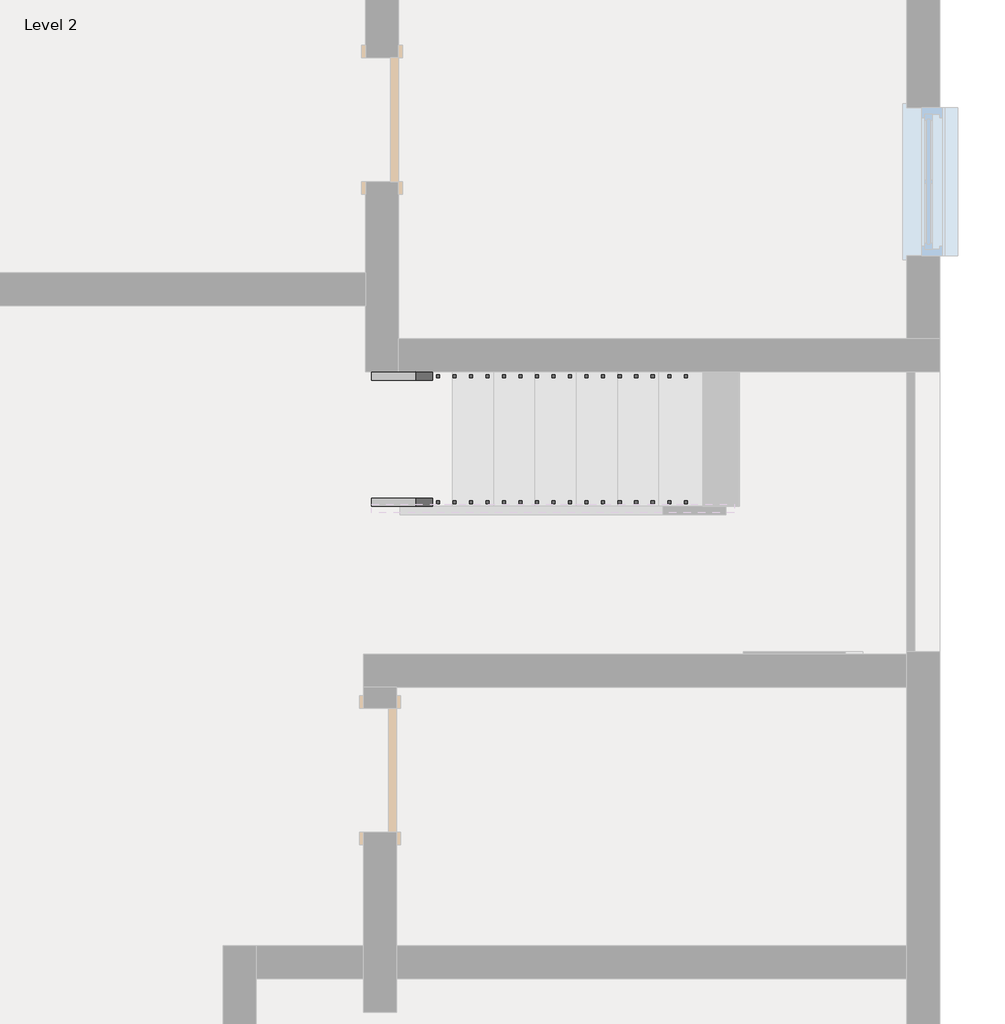
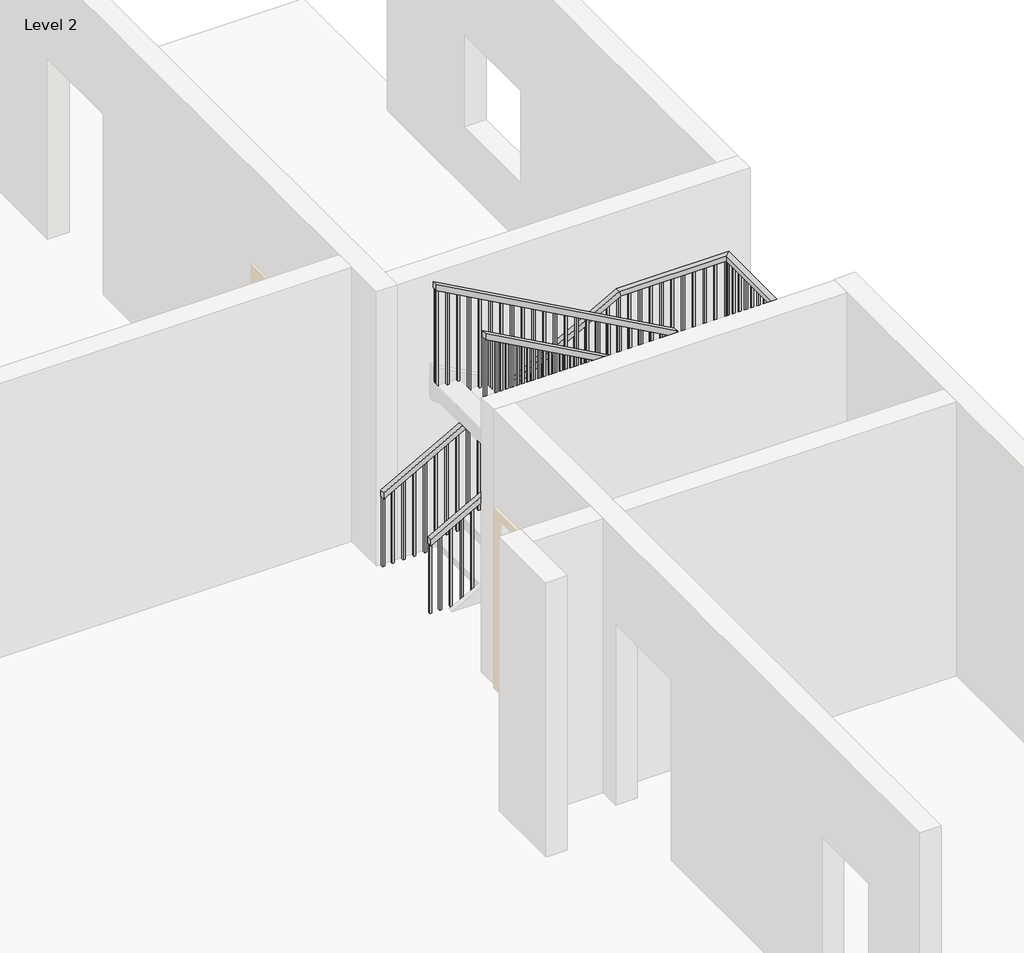
# One storey, part 3 of 4: 2 railings.
"""IFC4 building model written with IfcOpenShell, lengths in millimetres."""

from ifc_helpers import new_model, si_unit, frame, origin, place, context, project, spatial, polyline, outline, extrude, faceted_brep, element, save

model = new_model("IFC4")

# Units and contexts
model_context = context("Model", 3, world=origin())
ifc_project = project(units=[si_unit("LENGTHUNIT", "METRE", prefix="MILLI")], contexts=[model_context])

# Site, building, storey
site = spatial("IfcSite", under=ifc_project)
building = spatial("IfcBuilding", under=site)
storey = spatial("IfcBuildingStorey", under=building, Name="Level 2", Elevation=3048.0)

# Railings
placement = place(None, origin())
element("IfcRailing", 1, ObjectType="Handrail - Rectangular", at=placement, inside=storey, context=model_context, shape_type="SolidModel", body=[
    faceted_brep([(1537.1941283, 231.7547293, 4099.56), (1537.1941283, 231.7547293, 4041.4879132), (1537.1941283, 180.9547293, 4041.4879132), (1537.1941283, 180.9547293, 4099.56), (3765.8648053, 231.7547293, 5334.0), (3765.8648053, 180.9547293, 5334.0), (3765.8648053, 180.9547293, 5275.9279132), (3765.8648053, 231.7547293, 5275.9279132)], [[[0, 1, 2, 3]], [[4, 5, 6, 7]], [[1, 0, 4, 7]], [[2, 1, 7, 6]], [[3, 2, 6, 5]], [[0, 3, 5, 4]]]),
    faceted_brep([(3816.6648053, 231.7547293, 5334.0), (3816.6648053, 231.7547293, 5283.2), (3765.8648053, 231.7547293, 5283.2), (3765.8648053, 231.7547293, 5334.0), (3816.6648053, 142.8547293, 5334.0), (3765.8648053, 142.8547293, 5334.0), (3765.8648053, 92.0547293, 5283.2), (3816.6648053, 92.0547293, 5283.2)], [[[0, 1, 2, 3]], [[4, 5, 6, 7]], [[1, 0, 4, 7]], [[2, 1, 7, 6]], [[3, 2, 6, 5]], [[0, 3, 5, 4]]]),
    faceted_brep([(3816.6648053, 142.8547293, 5334.0), (3816.6648053, 92.0547293, 5283.2), (3765.8648053, 92.0547293, 5283.2), (3765.8648053, 142.8547293, 5334.0), (3816.6648053, 142.8547293, 5443.0223516), (3765.8648053, 142.8547293, 5413.0879132), (3765.8648053, 92.0547293, 5413.0879132), (3816.6648053, 92.0547293, 5443.0223516)], [[[0, 1, 2, 3]], [[4, 5, 6, 7]], [[1, 0, 4, 7]], [[2, 1, 7, 6]], [[3, 2, 6, 5]], [[0, 3, 5, 4]]]),
    faceted_brep([(3816.6648053, 92.0547293, 5443.0223516), (3765.8648053, 92.0547293, 5413.0879132), (3765.8648053, 142.8547293, 5413.0879132), (3816.6648053, 142.8547293, 5443.0223516), (1537.1941283, 92.0547293, 6705.6), (1537.1941283, 142.8547293, 6705.6), (1537.1941283, 142.8547293, 6647.5279132), (1537.1941283, 92.0547293, 6647.5279132)], [[[0, 1, 2, 3]], [[4, 5, 6, 7]], [[1, 0, 4, 7]], [[2, 1, 7, 6]], [[3, 2, 6, 5]], [[0, 3, 5, 4]]]),
    extrude(outline(polyline([(6631.7556667, 1565.5898053), (6642.3072849, 1546.5398053), (5654.04, 1546.5398053), (5654.04, 1565.5898053), (6631.7556667, 1565.5898053)])), frame((0.0, 107.9297293, 0.0), z_axis=(0.0, 1.0, 0.0), x_axis=(0.0, 0.0, 1.0)), (0.0, 0.0, 1.0), 19.05),
    extrude(outline(polyline([(6575.4803699, 1667.1898053), (6586.031988, 1648.1398053), (5654.04, 1648.1398053), (5654.04, 1667.1898053), (6575.4803699, 1667.1898053)])), frame((0.0, 107.9297293, 0.0), z_axis=(0.0, 1.0, 0.0), x_axis=(0.0, 0.0, 1.0)), (0.0, 0.0, 1.0), 19.05),
    extrude(outline(polyline([(6519.1609284, 1768.7898053), (6529.7125465, 1749.7398053), (5654.04, 1749.7398053), (5654.04, 1768.7898053), (6519.1609284, 1768.7898053)])), frame((0.0, 107.9297293, 0.0), z_axis=(0.0, 1.0, 0.0), x_axis=(0.0, 0.0, 1.0)), (0.0, 0.0, 1.0), 19.05),
    extrude(outline(polyline([(6462.9297761, 1870.3898053), (6473.4813943, 1851.3398053), (5516.88, 1851.3398053), (5516.88, 1870.3898053), (6462.9297761, 1870.3898053)])), frame((0.0, 107.9297293, 0.0), z_axis=(0.0, 1.0, 0.0), x_axis=(0.0, 0.0, 1.0)), (0.0, 0.0, 1.0), 19.05),
    extrude(outline(polyline([(6406.6544792, 1971.9898053), (6417.2060974, 1952.9398053), (5516.88, 1952.9398053), (5516.88, 1971.9898053), (6406.6544792, 1971.9898053)])), frame((0.0, 107.9297293, 0.0), z_axis=(0.0, 1.0, 0.0), x_axis=(0.0, 0.0, 1.0)), (0.0, 0.0, 1.0), 19.05),
    extrude(outline(polyline([(6350.3791823, 2073.5898053), (6360.9308005, 2054.5398053), (5379.72, 2054.5398053), (5379.72, 2073.5898053), (6350.3791823, 2073.5898053)])), frame((0.0, 107.9297293, 0.0), z_axis=(0.0, 1.0, 0.0), x_axis=(0.0, 0.0, 1.0)), (0.0, 0.0, 1.0), 19.05),
    extrude(outline(polyline([(6294.1038855, 2175.1898053), (6304.6555036, 2156.1398053), (5379.72, 2156.1398053), (5379.72, 2175.1898053), (6294.1038855, 2175.1898053)])), frame((0.0, 107.9297293, 0.0), z_axis=(0.0, 1.0, 0.0), x_axis=(0.0, 0.0, 1.0)), (0.0, 0.0, 1.0), 19.05),
    extrude(outline(polyline([(6237.8285886, 2276.7898053), (6248.3802067, 2257.7398053), (5379.72, 2257.7398053), (5379.72, 2276.7898053), (6237.8285886, 2276.7898053)])), frame((0.0, 107.9297293, 0.0), z_axis=(0.0, 1.0, 0.0), x_axis=(0.0, 0.0, 1.0)), (0.0, 0.0, 1.0), 19.05),
    extrude(outline(polyline([(6181.5532917, 2378.3898053), (6192.1049099, 2359.3398053), (5242.56, 2359.3398053), (5242.56, 2378.3898053), (6181.5532917, 2378.3898053)])), frame((0.0, 107.9297293, 0.0), z_axis=(0.0, 1.0, 0.0), x_axis=(0.0, 0.0, 1.0)), (0.0, 0.0, 1.0), 19.05),
    extrude(outline(polyline([(6125.2779948, 2479.9898053), (6135.829613, 2460.9398053), (5242.56, 2460.9398053), (5242.56, 2479.9898053), (6125.2779948, 2479.9898053)])), frame((0.0, 107.9297293, 0.0), z_axis=(0.0, 1.0, 0.0), x_axis=(0.0, 0.0, 1.0)), (0.0, 0.0, 1.0), 19.05),
    extrude(outline(polyline([(6069.0026979, 2581.5898053), (6079.5543161, 2562.5398053), (5105.4, 2562.5398053), (5105.4, 2581.5898053), (6069.0026979, 2581.5898053)])), frame((0.0, 107.9297293, 0.0), z_axis=(0.0, 1.0, 0.0), x_axis=(0.0, 0.0, 1.0)), (0.0, 0.0, 1.0), 19.05),
    extrude(outline(polyline([(6012.727401, 2683.1898053), (6023.2790192, 2664.1398053), (5105.4, 2664.1398053), (5105.4, 2683.1898053), (6012.727401, 2683.1898053)])), frame((0.0, 107.9297293, 0.0), z_axis=(0.0, 1.0, 0.0), x_axis=(0.0, 0.0, 1.0)), (0.0, 0.0, 1.0), 19.05),
    extrude(outline(polyline([(5956.4962488, 2784.7898053), (5967.0478669, 2765.7398053), (5105.4, 2765.7398053), (5105.4, 2784.7898053), (5956.4962488, 2784.7898053)])), frame((0.0, 107.9297293, 0.0), z_axis=(0.0, 1.0, 0.0), x_axis=(0.0, 0.0, 1.0)), (0.0, 0.0, 1.0), 19.05),
    extrude(outline(polyline([(5900.2209519, 2886.3898053), (5910.77257, 2867.3398053), (4968.24, 2867.3398053), (4968.24, 2886.3898053), (5900.2209519, 2886.3898053)])), frame((0.0, 107.9297293, 0.0), z_axis=(0.0, 1.0, 0.0), x_axis=(0.0, 0.0, 1.0)), (0.0, 0.0, 1.0), 19.05),
    extrude(outline(polyline([(5843.945655, 2987.9898053), (5854.4972732, 2968.9398053), (4968.24, 2968.9398053), (4968.24, 2987.9898053), (5843.945655, 2987.9898053)])), frame((0.0, 107.9297293, 0.0), z_axis=(0.0, 1.0, 0.0), x_axis=(0.0, 0.0, 1.0)), (0.0, 0.0, 1.0), 19.05),
    extrude(outline(polyline([(5787.6703581, 3089.5898053), (5798.2219763, 3070.5398053), (4831.08, 3070.5398053), (4831.08, 3089.5898053), (5787.6703581, 3089.5898053)])), frame((0.0, 107.9297293, 0.0), z_axis=(0.0, 1.0, 0.0), x_axis=(0.0, 0.0, 1.0)), (0.0, 0.0, 1.0), 19.05),
    extrude(outline(polyline([(5731.3950612, 3191.1898053), (5741.9466794, 3172.1398053), (4831.08, 3172.1398053), (4831.08, 3191.1898053), (5731.3950612, 3191.1898053)])), frame((0.0, 107.9297293, 0.0), z_axis=(0.0, 1.0, 0.0), x_axis=(0.0, 0.0, 1.0)), (0.0, 0.0, 1.0), 19.05),
    extrude(outline(polyline([(5675.1197643, 3292.7898053), (5685.6713825, 3273.7398053), (4831.08, 3273.7398053), (4831.08, 3292.7898053), (5675.1197643, 3292.7898053)])), frame((0.0, 107.9297293, 0.0), z_axis=(0.0, 1.0, 0.0), x_axis=(0.0, 0.0, 1.0)), (0.0, 0.0, 1.0), 19.05),
    extrude(outline(polyline([(5618.8444675, 3394.3898053), (5629.3960856, 3375.3398053), (4693.92, 3375.3398053), (4693.92, 3394.3898053), (5618.8444675, 3394.3898053)])), frame((0.0, 107.9297293, 0.0), z_axis=(0.0, 1.0, 0.0), x_axis=(0.0, 0.0, 1.0)), (0.0, 0.0, 1.0), 19.05),
    extrude(outline(polyline([(5562.5691706, 3495.9898053), (5573.1207888, 3476.9398053), (4693.92, 3476.9398053), (4693.92, 3495.9898053), (5562.5691706, 3495.9898053)])), frame((0.0, 107.9297293, 0.0), z_axis=(0.0, 1.0, 0.0), x_axis=(0.0, 0.0, 1.0)), (0.0, 0.0, 1.0), 19.05),
    extrude(outline(polyline([(5506.2938737, 3597.5898053), (5516.8454919, 3578.5398053), (4556.76, 3578.5398053), (4556.76, 3597.5898053), (5506.2938737, 3597.5898053)])), frame((0.0, 107.9297293, 0.0), z_axis=(0.0, 1.0, 0.0), x_axis=(0.0, 0.0, 1.0)), (0.0, 0.0, 1.0), 19.05),
    extrude(outline(polyline([(5450.0185768, 3699.1898053), (5460.570195, 3680.1398053), (4556.76, 3680.1398053), (4556.76, 3699.1898053), (5450.0185768, 3699.1898053)])), frame((0.0, 107.9297293, 0.0), z_axis=(0.0, 1.0, 0.0), x_axis=(0.0, 0.0, 1.0)), (0.0, 0.0, 1.0), 19.05),
    extrude(outline(polyline([(5284.8202537, 3781.9191283), (5274.2686355, 3762.8691283), (4419.6, 3762.8691283), (4419.6, 3781.9191283), (5284.8202537, 3781.9191283)])), frame((0.0, 196.8297293, 0.0), z_axis=(0.0, 1.0, 0.0), x_axis=(0.0, 0.0, 1.0)), (0.0, 0.0, 1.0), 19.05),
    extrude(outline(polyline([(5228.5449568, 3680.3191283), (5217.9933387, 3661.2691283), (4282.44, 3661.2691283), (4282.44, 3680.3191283), (5228.5449568, 3680.3191283)])), frame((0.0, 196.8297293, 0.0), z_axis=(0.0, 1.0, 0.0), x_axis=(0.0, 0.0, 1.0)), (0.0, 0.0, 1.0), 19.05),
    extrude(outline(polyline([(5172.2696599, 3578.7191283), (5161.7180418, 3559.6691283), (4282.44, 3559.6691283), (4282.44, 3578.7191283), (5172.2696599, 3578.7191283)])), frame((0.0, 196.8297293, 0.0), z_axis=(0.0, 1.0, 0.0), x_axis=(0.0, 0.0, 1.0)), (0.0, 0.0, 1.0), 19.05),
    extrude(outline(polyline([(5115.9943631, 3477.1191283), (5105.4427449, 3458.0691283), (4145.28, 3458.0691283), (4145.28, 3477.1191283), (5115.9943631, 3477.1191283)])), frame((0.0, 196.8297293, 0.0), z_axis=(0.0, 1.0, 0.0), x_axis=(0.0, 0.0, 1.0)), (0.0, 0.0, 1.0), 19.05),
    extrude(outline(polyline([(5059.7190662, 3375.5191283), (5049.167448, 3356.4691283), (4145.28, 3356.4691283), (4145.28, 3375.5191283), (5059.7190662, 3375.5191283)])), frame((0.0, 196.8297293, 0.0), z_axis=(0.0, 1.0, 0.0), x_axis=(0.0, 0.0, 1.0)), (0.0, 0.0, 1.0), 19.05),
    extrude(outline(polyline([(5003.4437693, 3273.9191283), (4992.8921511, 3254.8691283), (4008.12, 3254.8691283), (4008.12, 3273.9191283), (5003.4437693, 3273.9191283)])), frame((0.0, 196.8297293, 0.0), z_axis=(0.0, 1.0, 0.0), x_axis=(0.0, 0.0, 1.0)), (0.0, 0.0, 1.0), 19.05),
    extrude(outline(polyline([(4947.1684724, 3172.3191283), (4936.6168543, 3153.2691283), (4008.12, 3153.2691283), (4008.12, 3172.3191283), (4947.1684724, 3172.3191283)])), frame((0.0, 196.8297293, 0.0), z_axis=(0.0, 1.0, 0.0), x_axis=(0.0, 0.0, 1.0)), (0.0, 0.0, 1.0), 19.05),
    extrude(outline(polyline([(4890.8931755, 3070.7191283), (4880.3415574, 3051.6691283), (4008.12, 3051.6691283), (4008.12, 3070.7191283), (4890.8931755, 3070.7191283)])), frame((0.0, 196.8297293, 0.0), z_axis=(0.0, 1.0, 0.0), x_axis=(0.0, 0.0, 1.0)), (0.0, 0.0, 1.0), 19.05),
    extrude(outline(polyline([(4834.6178787, 2969.1191283), (4824.0662605, 2950.0691283), (3870.96, 2950.0691283), (3870.96, 2969.1191283), (4834.6178787, 2969.1191283)])), frame((0.0, 196.8297293, 0.0), z_axis=(0.0, 1.0, 0.0), x_axis=(0.0, 0.0, 1.0)), (0.0, 0.0, 1.0), 19.05),
    extrude(outline(polyline([(4778.3425818, 2867.5191283), (4767.7909636, 2848.4691283), (3870.96, 2848.4691283), (3870.96, 2867.5191283), (4778.3425818, 2867.5191283)])), frame((0.0, 196.8297293, 0.0), z_axis=(0.0, 1.0, 0.0), x_axis=(0.0, 0.0, 1.0)), (0.0, 0.0, 1.0), 19.05),
    extrude(outline(polyline([(4722.0672849, 2765.9191283), (4711.5156667, 2746.8691283), (3733.8, 2746.8691283), (3733.8, 2765.9191283), (4722.0672849, 2765.9191283)])), frame((0.0, 196.8297293, 0.0), z_axis=(0.0, 1.0, 0.0), x_axis=(0.0, 0.0, 1.0)), (0.0, 0.0, 1.0), 19.05),
    extrude(outline(polyline([(4665.791988, 2664.3191283), (4655.2403699, 2645.2691283), (3733.8, 2645.2691283), (3733.8, 2664.3191283), (4665.791988, 2664.3191283)])), frame((0.0, 196.8297293, 0.0), z_axis=(0.0, 1.0, 0.0), x_axis=(0.0, 0.0, 1.0)), (0.0, 0.0, 1.0), 19.05),
    extrude(outline(polyline([(4609.4725465, 2562.7191283), (4598.9209284, 2543.6691283), (3733.8, 2543.6691283), (3733.8, 2562.7191283), (4609.4725465, 2562.7191283)])), frame((0.0, 196.8297293, 0.0), z_axis=(0.0, 1.0, 0.0), x_axis=(0.0, 0.0, 1.0)), (0.0, 0.0, 1.0), 19.05),
    extrude(outline(polyline([(4553.2413943, 2461.1191283), (4542.6897761, 2442.0691283), (3596.64, 2442.0691283), (3596.64, 2461.1191283), (4553.2413943, 2461.1191283)])), frame((0.0, 196.8297293, 0.0), z_axis=(0.0, 1.0, 0.0), x_axis=(0.0, 0.0, 1.0)), (0.0, 0.0, 1.0), 19.05),
    extrude(outline(polyline([(4496.9660974, 2359.5191283), (4486.4144792, 2340.4691283), (3596.64, 2340.4691283), (3596.64, 2359.5191283), (4496.9660974, 2359.5191283)])), frame((0.0, 196.8297293, 0.0), z_axis=(0.0, 1.0, 0.0), x_axis=(0.0, 0.0, 1.0)), (0.0, 0.0, 1.0), 19.05),
    extrude(outline(polyline([(4440.6908005, 2257.9191283), (4430.1391823, 2238.8691283), (3459.48, 2238.8691283), (3459.48, 2257.9191283), (4440.6908005, 2257.9191283)])), frame((0.0, 196.8297293, 0.0), z_axis=(0.0, 1.0, 0.0), x_axis=(0.0, 0.0, 1.0)), (0.0, 0.0, 1.0), 19.05),
    extrude(outline(polyline([(4384.4155036, 2156.3191283), (4373.8638855, 2137.2691283), (3459.48, 2137.2691283), (3459.48, 2156.3191283), (4384.4155036, 2156.3191283)])), frame((0.0, 196.8297293, 0.0), z_axis=(0.0, 1.0, 0.0), x_axis=(0.0, 0.0, 1.0)), (0.0, 0.0, 1.0), 19.05),
    extrude(outline(polyline([(4328.1402067, 2054.7191283), (4317.5885886, 2035.6691283), (3459.48, 2035.6691283), (3459.48, 2054.7191283), (4328.1402067, 2054.7191283)])), frame((0.0, 196.8297293, 0.0), z_axis=(0.0, 1.0, 0.0), x_axis=(0.0, 0.0, 1.0)), (0.0, 0.0, 1.0), 19.05),
    extrude(outline(polyline([(4271.8649099, 1953.1191283), (4261.3132917, 1934.0691283), (3322.32, 1934.0691283), (3322.32, 1953.1191283), (4271.8649099, 1953.1191283)])), frame((0.0, 196.8297293, 0.0), z_axis=(0.0, 1.0, 0.0), x_axis=(0.0, 0.0, 1.0)), (0.0, 0.0, 1.0), 19.05),
    extrude(outline(polyline([(4215.589613, 1851.5191283), (4205.0379948, 1832.4691283), (3322.32, 1832.4691283), (3322.32, 1851.5191283), (4215.589613, 1851.5191283)])), frame((0.0, 196.8297293, 0.0), z_axis=(0.0, 1.0, 0.0), x_axis=(0.0, 0.0, 1.0)), (0.0, 0.0, 1.0), 19.05),
    extrude(outline(polyline([(4159.3143161, 1749.9191283), (4148.7626979, 1730.8691283), (3185.16, 1730.8691283), (3185.16, 1749.9191283), (4159.3143161, 1749.9191283)])), frame((0.0, 196.8297293, 0.0), z_axis=(0.0, 1.0, 0.0), x_axis=(0.0, 0.0, 1.0)), (0.0, 0.0, 1.0), 19.05),
    extrude(outline(polyline([(4103.0390192, 1648.3191283), (4092.487401, 1629.2691283), (3185.16, 1629.2691283), (3185.16, 1648.3191283), (4103.0390192, 1648.3191283)])), frame((0.0, 196.8297293, 0.0), z_axis=(0.0, 1.0, 0.0), x_axis=(0.0, 0.0, 1.0)), (0.0, 0.0, 1.0), 19.05),
    extrude(outline(polyline([(3781.7398053, 126.9797293), (3800.7898053, 126.9797293), (3800.7898053, 107.9297293), (3781.7398053, 107.9297293), (3781.7398053, 126.9797293)])), frame((0.0, 0.0, 4419.6), z_axis=(0.0, 0.0, 1.0), x_axis=(1.0, 0.0, 0.0)), (0.0, 0.0, 1.0), 863.6),
    extrude(outline(polyline([(5295.2725465, 3800.7898053), (5284.7209284, 3781.7398053), (4419.6, 3781.7398053), (4419.6, 3800.7898053), (5295.2725465, 3800.7898053)])), frame((0.0, 196.8297293, 0.0), z_axis=(0.0, 1.0, 0.0), x_axis=(0.0, 0.0, 1.0)), (0.0, 0.0, 1.0), 19.05),
    extrude(outline(polyline([(6636.9762951, 1556.2441283), (6647.5279132, 1537.1941283), (5654.04, 1537.1941283), (5654.04, 1556.2441283), (6636.9762951, 1556.2441283)])), frame((0.0, 107.9297293, 0.0), z_axis=(0.0, 1.0, 0.0), x_axis=(0.0, 0.0, 1.0)), (0.0, 0.0, 1.0), 19.05),
    extrude(outline(polyline([(4052.0395314, 1556.2441283), (4041.4879132, 1537.1941283), (3185.16, 1537.1941283), (3185.16, 1556.2441283), (4052.0395314, 1556.2441283)])), frame((0.0, 196.8297293, 0.0), z_axis=(0.0, 1.0, 0.0), x_axis=(0.0, 0.0, 1.0)), (0.0, 0.0, 1.0), 19.05),
])
element("IfcRailing", 2, ObjectType="Handrail - Rectangular", at=placement, inside=storey, context=model_context, shape_type="SolidModel", body=[
    faceted_brep([(1537.1941283, 1006.4547293, 4099.56), (1537.1941283, 1006.4547293, 4041.4879132), (1537.1941283, 955.6547293, 4041.4879132), (1537.1941283, 955.6547293, 4099.56), (3765.8648053, 1006.4547293, 5334.0), (3778.9939056, 1006.4547293, 5283.2), (3778.9939056, 955.6547293, 5283.2), (3765.8648053, 955.6547293, 5334.0), (4826.4941283, 1006.4547293, 5334.0), (4826.4941283, 1006.4547293, 5283.2), (4775.6941283, 955.6547293, 5283.2), (4775.6941283, 955.6547293, 5334.0), (4826.4941283, -714.2964201, 5334.0), (4826.4941283, -714.2964201, 5283.2), (4775.6941283, -663.4964201, 5283.2), (4775.6941283, -663.4964201, 5334.0), (4013.4948805, -714.2964201, 5334.0), (4000.3657803, -714.2964201, 5283.2), (4000.3657803, -663.4964201, 5283.2), (4013.4948805, -663.4964201, 5334.0), (1537.1941283, -714.2964201, 6705.6), (1537.1941283, -663.4964201, 6705.6), (1537.1941283, -663.4964201, 6647.5279132), (1537.1941283, -714.2964201, 6647.5279132)], [[[0, 1, 2, 3]], [[1, 0, 4, 5]], [[2, 1, 5, 6]], [[3, 2, 6, 7]], [[0, 3, 7, 4]], [[5, 4, 8, 9]], [[6, 5, 9, 10]], [[7, 6, 10, 11]], [[4, 7, 11, 8]], [[9, 8, 12, 13]], [[10, 9, 13, 14]], [[11, 10, 14, 15]], [[8, 11, 15, 12]], [[13, 12, 16, 17]], [[14, 13, 17, 18]], [[15, 14, 18, 19]], [[12, 15, 19, 16]], [[20, 21, 22, 23]], [[17, 16, 20, 23]], [[18, 17, 23, 22]], [[19, 18, 22, 21]], [[16, 19, 21, 20]]]),
    extrude(outline(polyline([(6645.7693102, 1540.3691283), (5654.04, 1540.3691283), (5654.04, 1559.4191283), (6635.2176921, 1559.4191283), (6645.7693102, 1540.3691283)])), frame((0.0, -698.4214201, 0.0), z_axis=(0.0, 1.0, 0.0), x_axis=(0.0, 0.0, 1.0)), (0.0, 0.0, 1.0), 19.05),
    extrude(outline(polyline([(6589.4940133, 1641.9691283), (5654.04, 1641.9691283), (5654.04, 1661.0191283), (6578.9423952, 1661.0191283), (6589.4940133, 1641.9691283)])), frame((0.0, -698.4214201, 0.0), z_axis=(0.0, 1.0, 0.0), x_axis=(0.0, 0.0, 1.0)), (0.0, 0.0, 1.0), 19.05),
    extrude(outline(polyline([(6533.2187165, 1743.5691283), (5654.04, 1743.5691283), (5654.04, 1762.6191283), (6522.6670983, 1762.6191283), (6533.2187165, 1743.5691283)])), frame((0.0, -698.4214201, 0.0), z_axis=(0.0, 1.0, 0.0), x_axis=(0.0, 0.0, 1.0)), (0.0, 0.0, 1.0), 19.05),
    extrude(outline(polyline([(6476.9434196, 1845.1691283), (5516.88, 1845.1691283), (5516.88, 1864.2191283), (6466.3918014, 1864.2191283), (6476.9434196, 1845.1691283)])), frame((0.0, -698.4214201, 0.0), z_axis=(0.0, 1.0, 0.0), x_axis=(0.0, 0.0, 1.0)), (0.0, 0.0, 1.0), 19.05),
    extrude(outline(polyline([(6420.6681227, 1946.7691283), (5516.88, 1946.7691283), (5516.88, 1965.8191283), (6410.1165045, 1965.8191283), (6420.6681227, 1946.7691283)])), frame((0.0, -698.4214201, 0.0), z_axis=(0.0, 1.0, 0.0), x_axis=(0.0, 0.0, 1.0)), (0.0, 0.0, 1.0), 19.05),
    extrude(outline(polyline([(6364.3928258, 2048.3691283), (5379.72, 2048.3691283), (5379.72, 2067.4191283), (6353.8412076, 2067.4191283), (6364.3928258, 2048.3691283)])), frame((0.0, -698.4214201, 0.0), z_axis=(0.0, 1.0, 0.0), x_axis=(0.0, 0.0, 1.0)), (0.0, 0.0, 1.0), 19.05),
    extrude(outline(polyline([(6308.1175289, 2149.9691283), (5379.72, 2149.9691283), (5379.72, 2169.0191283), (6297.5659108, 2169.0191283), (6308.1175289, 2149.9691283)])), frame((0.0, -698.4214201, 0.0), z_axis=(0.0, 1.0, 0.0), x_axis=(0.0, 0.0, 1.0)), (0.0, 0.0, 1.0), 19.05),
    extrude(outline(polyline([(6251.8422321, 2251.5691283), (5379.72, 2251.5691283), (5379.72, 2270.6191283), (6241.2906139, 2270.6191283), (6251.8422321, 2251.5691283)])), frame((0.0, -698.4214201, 0.0), z_axis=(0.0, 1.0, 0.0), x_axis=(0.0, 0.0, 1.0)), (0.0, 0.0, 1.0), 19.05),
    extrude(outline(polyline([(6195.5669352, 2353.1691283), (5242.56, 2353.1691283), (5242.56, 2372.2191283), (6185.015317, 2372.2191283), (6195.5669352, 2353.1691283)])), frame((0.0, -698.4214201, 0.0), z_axis=(0.0, 1.0, 0.0), x_axis=(0.0, 0.0, 1.0)), (0.0, 0.0, 1.0), 19.05),
    extrude(outline(polyline([(6139.2916383, 2454.7691283), (5242.56, 2454.7691283), (5242.56, 2473.8191283), (6128.7400201, 2473.8191283), (6139.2916383, 2454.7691283)])), frame((0.0, -698.4214201, 0.0), z_axis=(0.0, 1.0, 0.0), x_axis=(0.0, 0.0, 1.0)), (0.0, 0.0, 1.0), 19.05),
    extrude(outline(polyline([(6083.0163414, 2556.3691283), (5105.4, 2556.3691283), (5105.4, 2575.4191283), (6072.4647232, 2575.4191283), (6083.0163414, 2556.3691283)])), frame((0.0, -698.4214201, 0.0), z_axis=(0.0, 1.0, 0.0), x_axis=(0.0, 0.0, 1.0)), (0.0, 0.0, 1.0), 19.05),
    extrude(outline(polyline([(6026.7410445, 2657.9691283), (5105.4, 2657.9691283), (5105.4, 2677.0191283), (6016.1894264, 2677.0191283), (6026.7410445, 2657.9691283)])), frame((0.0, -698.4214201, 0.0), z_axis=(0.0, 1.0, 0.0), x_axis=(0.0, 0.0, 1.0)), (0.0, 0.0, 1.0), 19.05),
    extrude(outline(polyline([(5970.4657476, 2759.5691283), (5105.4, 2759.5691283), (5105.4, 2778.6191283), (5959.9141295, 2778.6191283), (5970.4657476, 2759.5691283)])), frame((0.0, -698.4214201, 0.0), z_axis=(0.0, 1.0, 0.0), x_axis=(0.0, 0.0, 1.0)), (0.0, 0.0, 1.0), 19.05),
    extrude(outline(polyline([(5914.3449568, 2861.1691283), (4968.24, 2861.1691283), (4968.24, 2880.2191283), (5903.7933387, 2880.2191283), (5914.3449568, 2861.1691283)])), frame((0.0, -698.4214201, 0.0), z_axis=(0.0, 1.0, 0.0), x_axis=(0.0, 0.0, 1.0)), (0.0, 0.0, 1.0), 19.05),
    extrude(outline(polyline([(5858.0696599, 2962.7691283), (4968.24, 2962.7691283), (4968.24, 2981.8191283), (5847.5180418, 2981.8191283), (5858.0696599, 2962.7691283)])), frame((0.0, -698.4214201, 0.0), z_axis=(0.0, 1.0, 0.0), x_axis=(0.0, 0.0, 1.0)), (0.0, 0.0, 1.0), 19.05),
    extrude(outline(polyline([(5801.7943631, 3064.3691283), (4831.08, 3064.3691283), (4831.08, 3083.4191283), (5791.2427449, 3083.4191283), (5801.7943631, 3064.3691283)])), frame((0.0, -698.4214201, 0.0), z_axis=(0.0, 1.0, 0.0), x_axis=(0.0, 0.0, 1.0)), (0.0, 0.0, 1.0), 19.05),
    extrude(outline(polyline([(5745.5190662, 3165.9691283), (4831.08, 3165.9691283), (4831.08, 3185.0191283), (5734.967448, 3185.0191283), (5745.5190662, 3165.9691283)])), frame((0.0, -698.4214201, 0.0), z_axis=(0.0, 1.0, 0.0), x_axis=(0.0, 0.0, 1.0)), (0.0, 0.0, 1.0), 19.05),
    extrude(outline(polyline([(5689.0892632, 3267.5691283), (4831.08, 3267.5691283), (4831.08, 3286.6191283), (5678.5376451, 3286.6191283), (5689.0892632, 3267.5691283)])), frame((0.0, -698.4214201, 0.0), z_axis=(0.0, 1.0, 0.0), x_axis=(0.0, 0.0, 1.0)), (0.0, 0.0, 1.0), 19.05),
    extrude(outline(polyline([(5632.9684724, 3369.1691283), (4693.92, 3369.1691283), (4693.92, 3388.2191283), (5622.4168543, 3388.2191283), (5632.9684724, 3369.1691283)])), frame((0.0, -698.4214201, 0.0), z_axis=(0.0, 1.0, 0.0), x_axis=(0.0, 0.0, 1.0)), (0.0, 0.0, 1.0), 19.05),
    extrude(outline(polyline([(5576.6931755, 3470.7691283), (4693.92, 3470.7691283), (4693.92, 3489.8191283), (5566.1415574, 3489.8191283), (5576.6931755, 3470.7691283)])), frame((0.0, -698.4214201, 0.0), z_axis=(0.0, 1.0, 0.0), x_axis=(0.0, 0.0, 1.0)), (0.0, 0.0, 1.0), 19.05),
    extrude(outline(polyline([(5520.4178787, 3572.3691283), (4556.76, 3572.3691283), (4556.76, 3591.4191283), (5509.8662605, 3591.4191283), (5520.4178787, 3572.3691283)])), frame((0.0, -698.4214201, 0.0), z_axis=(0.0, 1.0, 0.0), x_axis=(0.0, 0.0, 1.0)), (0.0, 0.0, 1.0), 19.05),
    extrude(outline(polyline([(5464.1425818, 3673.9691283), (4556.76, 3673.9691283), (4556.76, 3693.0191283), (5453.5909636, 3693.0191283), (5464.1425818, 3673.9691283)])), frame((0.0, -698.4214201, 0.0), z_axis=(0.0, 1.0, 0.0), x_axis=(0.0, 0.0, 1.0)), (0.0, 0.0, 1.0), 19.05),
    extrude(outline(polyline([(5407.8672849, 3775.5691283), (4419.6, 3775.5691283), (4419.6, 3794.6191283), (5397.3156667, 3794.6191283), (5407.8672849, 3775.5691283)])), frame((0.0, -698.4214201, 0.0), z_axis=(0.0, 1.0, 0.0), x_axis=(0.0, 0.0, 1.0)), (0.0, 0.0, 1.0), 19.05),
    extrude(outline(polyline([(5351.591988, 3877.1691283), (4419.6, 3877.1691283), (4419.6, 3896.2191283), (5341.0403699, 3896.2191283), (5351.591988, 3877.1691283)])), frame((0.0, -698.4214201, 0.0), z_axis=(0.0, 1.0, 0.0), x_axis=(0.0, 0.0, 1.0)), (0.0, 0.0, 1.0), 19.05),
    extrude(outline(polyline([(5295.3166911, 3978.7691283), (4419.6, 3978.7691283), (4419.6, 3997.8191283), (5284.765073, 3997.8191283), (5295.3166911, 3978.7691283)])), frame((0.0, -698.4214201, 0.0), z_axis=(0.0, 1.0, 0.0), x_axis=(0.0, 0.0, 1.0)), (0.0, 0.0, 1.0), 19.05),
    extrude(outline(polyline([(4099.4191283, -698.4214201), (4080.3691283, -698.4214201), (4080.3691283, -679.3714201), (4099.4191283, -679.3714201), (4099.4191283, -698.4214201)])), frame((0.0, 0.0, 4419.6), z_axis=(0.0, 0.0, 1.0), x_axis=(1.0, 0.0, 0.0)), (0.0, 0.0, 1.0), 863.6),
    extrude(outline(polyline([(4201.0191283, -698.4214201), (4181.9691283, -698.4214201), (4181.9691283, -679.3714201), (4201.0191283, -679.3714201), (4201.0191283, -698.4214201)])), frame((0.0, 0.0, 4419.6), z_axis=(0.0, 0.0, 1.0), x_axis=(1.0, 0.0, 0.0)), (0.0, 0.0, 1.0), 863.6),
    extrude(outline(polyline([(4302.6191283, -698.4214201), (4283.5691283, -698.4214201), (4283.5691283, -679.3714201), (4302.6191283, -679.3714201), (4302.6191283, -698.4214201)])), frame((0.0, 0.0, 4419.6), z_axis=(0.0, 0.0, 1.0), x_axis=(1.0, 0.0, 0.0)), (0.0, 0.0, 1.0), 863.6),
    extrude(outline(polyline([(4404.2191283, -698.4214201), (4385.1691283, -698.4214201), (4385.1691283, -679.3714201), (4404.2191283, -679.3714201), (4404.2191283, -698.4214201)])), frame((0.0, 0.0, 4419.6), z_axis=(0.0, 0.0, 1.0), x_axis=(1.0, 0.0, 0.0)), (0.0, 0.0, 1.0), 863.6),
    extrude(outline(polyline([(4505.8191283, -698.4214201), (4486.7691283, -698.4214201), (4486.7691283, -679.3714201), (4505.8191283, -679.3714201), (4505.8191283, -698.4214201)])), frame((0.0, 0.0, 4419.6), z_axis=(0.0, 0.0, 1.0), x_axis=(1.0, 0.0, 0.0)), (0.0, 0.0, 1.0), 863.6),
    extrude(outline(polyline([(4607.4191283, -698.4214201), (4588.3691283, -698.4214201), (4588.3691283, -679.3714201), (4607.4191283, -679.3714201), (4607.4191283, -698.4214201)])), frame((0.0, 0.0, 4419.6), z_axis=(0.0, 0.0, 1.0), x_axis=(1.0, 0.0, 0.0)), (0.0, 0.0, 1.0), 863.6),
    extrude(outline(polyline([(4709.0191283, -698.4214201), (4689.9691283, -698.4214201), (4689.9691283, -679.3714201), (4709.0191283, -679.3714201), (4709.0191283, -698.4214201)])), frame((0.0, 0.0, 4419.6), z_axis=(0.0, 0.0, 1.0), x_axis=(1.0, 0.0, 0.0)), (0.0, 0.0, 1.0), 863.6),
    extrude(outline(polyline([(4810.6191283, -635.0202707), (4810.6191283, -654.0702707), (4791.5691283, -654.0702707), (4791.5691283, -635.0202707), (4810.6191283, -635.0202707)])), frame((0.0, 0.0, 4419.6), z_axis=(0.0, 0.0, 1.0), x_axis=(1.0, 0.0, 0.0)), (0.0, 0.0, 1.0), 863.6),
    extrude(outline(polyline([(4810.6191283, -533.4202707), (4810.6191283, -552.4702707), (4791.5691283, -552.4702707), (4791.5691283, -533.4202707), (4810.6191283, -533.4202707)])), frame((0.0, 0.0, 4419.6), z_axis=(0.0, 0.0, 1.0), x_axis=(1.0, 0.0, 0.0)), (0.0, 0.0, 1.0), 863.6),
    extrude(outline(polyline([(4810.6191283, -431.8202707), (4810.6191283, -450.8702707), (4791.5691283, -450.8702707), (4791.5691283, -431.8202707), (4810.6191283, -431.8202707)])), frame((0.0, 0.0, 4419.6), z_axis=(0.0, 0.0, 1.0), x_axis=(1.0, 0.0, 0.0)), (0.0, 0.0, 1.0), 863.6),
    extrude(outline(polyline([(4810.6191283, -330.2202707), (4810.6191283, -349.2702707), (4791.5691283, -349.2702707), (4791.5691283, -330.2202707), (4810.6191283, -330.2202707)])), frame((0.0, 0.0, 4419.6), z_axis=(0.0, 0.0, 1.0), x_axis=(1.0, 0.0, 0.0)), (0.0, 0.0, 1.0), 863.6),
    extrude(outline(polyline([(4810.6191283, -228.6202707), (4810.6191283, -247.6702707), (4791.5691283, -247.6702707), (4791.5691283, -228.6202707), (4810.6191283, -228.6202707)])), frame((0.0, 0.0, 4419.6), z_axis=(0.0, 0.0, 1.0), x_axis=(1.0, 0.0, 0.0)), (0.0, 0.0, 1.0), 863.6),
    extrude(outline(polyline([(4810.6191283, -127.0202707), (4810.6191283, -146.0702707), (4791.5691283, -146.0702707), (4791.5691283, -127.0202707), (4810.6191283, -127.0202707)])), frame((0.0, 0.0, 4419.6), z_axis=(0.0, 0.0, 1.0), x_axis=(1.0, 0.0, 0.0)), (0.0, 0.0, 1.0), 863.6),
    extrude(outline(polyline([(4810.6191283, -25.4202707), (4810.6191283, -44.4702707), (4791.5691283, -44.4702707), (4791.5691283, -25.4202707), (4810.6191283, -25.4202707)])), frame((0.0, 0.0, 4419.6), z_axis=(0.0, 0.0, 1.0), x_axis=(1.0, 0.0, 0.0)), (0.0, 0.0, 1.0), 863.6),
    extrude(outline(polyline([(4810.6191283, 76.1797293), (4810.6191283, 57.1297293), (4791.5691283, 57.1297293), (4791.5691283, 76.1797293), (4810.6191283, 76.1797293)])), frame((0.0, 0.0, 4419.6), z_axis=(0.0, 0.0, 1.0), x_axis=(1.0, 0.0, 0.0)), (0.0, 0.0, 1.0), 863.6),
    extrude(outline(polyline([(4810.6191283, 177.7797293), (4810.6191283, 158.7297293), (4791.5691283, 158.7297293), (4791.5691283, 177.7797293), (4810.6191283, 177.7797293)])), frame((0.0, 0.0, 4419.6), z_axis=(0.0, 0.0, 1.0), x_axis=(1.0, 0.0, 0.0)), (0.0, 0.0, 1.0), 863.6),
    extrude(outline(polyline([(4810.6191283, 279.3797293), (4810.6191283, 260.3297293), (4791.5691283, 260.3297293), (4791.5691283, 279.3797293), (4810.6191283, 279.3797293)])), frame((0.0, 0.0, 4419.6), z_axis=(0.0, 0.0, 1.0), x_axis=(1.0, 0.0, 0.0)), (0.0, 0.0, 1.0), 863.6),
    extrude(outline(polyline([(4810.6191283, 380.9797293), (4810.6191283, 361.9297293), (4791.5691283, 361.9297293), (4791.5691283, 380.9797293), (4810.6191283, 380.9797293)])), frame((0.0, 0.0, 4419.6), z_axis=(0.0, 0.0, 1.0), x_axis=(1.0, 0.0, 0.0)), (0.0, 0.0, 1.0), 863.6),
    extrude(outline(polyline([(4810.6191283, 482.5797293), (4810.6191283, 463.5297293), (4791.5691283, 463.5297293), (4791.5691283, 482.5797293), (4810.6191283, 482.5797293)])), frame((0.0, 0.0, 4419.6), z_axis=(0.0, 0.0, 1.0), x_axis=(1.0, 0.0, 0.0)), (0.0, 0.0, 1.0), 863.6),
    extrude(outline(polyline([(4810.6191283, 584.1797293), (4810.6191283, 565.1297293), (4791.5691283, 565.1297293), (4791.5691283, 584.1797293), (4810.6191283, 584.1797293)])), frame((0.0, 0.0, 4419.6), z_axis=(0.0, 0.0, 1.0), x_axis=(1.0, 0.0, 0.0)), (0.0, 0.0, 1.0), 863.6),
    extrude(outline(polyline([(4810.6191283, 685.7797293), (4810.6191283, 666.7297293), (4791.5691283, 666.7297293), (4791.5691283, 685.7797293), (4810.6191283, 685.7797293)])), frame((0.0, 0.0, 4419.6), z_axis=(0.0, 0.0, 1.0), x_axis=(1.0, 0.0, 0.0)), (0.0, 0.0, 1.0), 863.6),
    extrude(outline(polyline([(4810.6191283, 787.3797293), (4810.6191283, 768.3297293), (4791.5691283, 768.3297293), (4791.5691283, 787.3797293), (4810.6191283, 787.3797293)])), frame((0.0, 0.0, 4419.6), z_axis=(0.0, 0.0, 1.0), x_axis=(1.0, 0.0, 0.0)), (0.0, 0.0, 1.0), 863.6),
    extrude(outline(polyline([(4810.6191283, 888.9797293), (4810.6191283, 869.9297293), (4791.5691283, 869.9297293), (4791.5691283, 888.9797293), (4810.6191283, 888.9797293)])), frame((0.0, 0.0, 4419.6), z_axis=(0.0, 0.0, 1.0), x_axis=(1.0, 0.0, 0.0)), (0.0, 0.0, 1.0), 863.6),
    extrude(outline(polyline([(4778.8691283, 990.5797293), (4797.9191283, 990.5797293), (4797.9191283, 971.5297293), (4778.8691283, 971.5297293), (4778.8691283, 990.5797293)])), frame((0.0, 0.0, 4419.6), z_axis=(0.0, 0.0, 1.0), x_axis=(1.0, 0.0, 0.0)), (0.0, 0.0, 1.0), 863.6),
    extrude(outline(polyline([(4677.2691283, 990.5797293), (4696.3191283, 990.5797293), (4696.3191283, 971.5297293), (4677.2691283, 971.5297293), (4677.2691283, 990.5797293)])), frame((0.0, 0.0, 4419.6), z_axis=(0.0, 0.0, 1.0), x_axis=(1.0, 0.0, 0.0)), (0.0, 0.0, 1.0), 863.6),
    extrude(outline(polyline([(4575.6691283, 990.5797293), (4594.7191283, 990.5797293), (4594.7191283, 971.5297293), (4575.6691283, 971.5297293), (4575.6691283, 990.5797293)])), frame((0.0, 0.0, 4419.6), z_axis=(0.0, 0.0, 1.0), x_axis=(1.0, 0.0, 0.0)), (0.0, 0.0, 1.0), 863.6),
    extrude(outline(polyline([(4474.0691283, 990.5797293), (4493.1191283, 990.5797293), (4493.1191283, 971.5297293), (4474.0691283, 971.5297293), (4474.0691283, 990.5797293)])), frame((0.0, 0.0, 4419.6), z_axis=(0.0, 0.0, 1.0), x_axis=(1.0, 0.0, 0.0)), (0.0, 0.0, 1.0), 863.6),
    extrude(outline(polyline([(4372.4691283, 990.5797293), (4391.5191283, 990.5797293), (4391.5191283, 971.5297293), (4372.4691283, 971.5297293), (4372.4691283, 990.5797293)])), frame((0.0, 0.0, 4419.6), z_axis=(0.0, 0.0, 1.0), x_axis=(1.0, 0.0, 0.0)), (0.0, 0.0, 1.0), 863.6),
    extrude(outline(polyline([(4270.8691283, 990.5797293), (4289.9191283, 990.5797293), (4289.9191283, 971.5297293), (4270.8691283, 971.5297293), (4270.8691283, 990.5797293)])), frame((0.0, 0.0, 4419.6), z_axis=(0.0, 0.0, 1.0), x_axis=(1.0, 0.0, 0.0)), (0.0, 0.0, 1.0), 863.6),
    extrude(outline(polyline([(4169.2691283, 990.5797293), (4188.3191283, 990.5797293), (4188.3191283, 971.5297293), (4169.2691283, 971.5297293), (4169.2691283, 990.5797293)])), frame((0.0, 0.0, 4419.6), z_axis=(0.0, 0.0, 1.0), x_axis=(1.0, 0.0, 0.0)), (0.0, 0.0, 1.0), 863.6),
    extrude(outline(polyline([(4067.6691283, 990.5797293), (4086.7191283, 990.5797293), (4086.7191283, 971.5297293), (4067.6691283, 971.5297293), (4067.6691283, 990.5797293)])), frame((0.0, 0.0, 4419.6), z_axis=(0.0, 0.0, 1.0), x_axis=(1.0, 0.0, 0.0)), (0.0, 0.0, 1.0), 863.6),
    extrude(outline(polyline([(3966.0691283, 990.5797293), (3985.1191283, 990.5797293), (3985.1191283, 971.5297293), (3966.0691283, 971.5297293), (3966.0691283, 990.5797293)])), frame((0.0, 0.0, 4419.6), z_axis=(0.0, 0.0, 1.0), x_axis=(1.0, 0.0, 0.0)), (0.0, 0.0, 1.0), 863.6),
    extrude(outline(polyline([(3864.4691283, 990.5797293), (3883.5191283, 990.5797293), (3883.5191283, 971.5297293), (3864.4691283, 971.5297293), (3864.4691283, 990.5797293)])), frame((0.0, 0.0, 4419.6), z_axis=(0.0, 0.0, 1.0), x_axis=(1.0, 0.0, 0.0)), (0.0, 0.0, 1.0), 863.6),
    extrude(outline(polyline([(3762.8691283, 990.5797293), (3781.9191283, 990.5797293), (3781.9191283, 971.5297293), (3762.8691283, 971.5297293), (3762.8691283, 990.5797293)])), frame((0.0, 0.0, 4419.6), z_axis=(0.0, 0.0, 1.0), x_axis=(1.0, 0.0, 0.0)), (0.0, 0.0, 1.0), 863.6),
    extrude(outline(polyline([(5217.9933387, 3661.2691283), (4282.44, 3661.2691283), (4282.44, 3680.3191283), (5228.5449568, 3680.3191283), (5217.9933387, 3661.2691283)])), frame((0.0, 971.5297293, 0.0), z_axis=(0.0, 1.0, 0.0), x_axis=(0.0, 0.0, 1.0)), (0.0, 0.0, 1.0), 19.05),
    extrude(outline(polyline([(5161.7180418, 3559.6691283), (4282.44, 3559.6691283), (4282.44, 3578.7191283), (5172.2696599, 3578.7191283), (5161.7180418, 3559.6691283)])), frame((0.0, 971.5297293, 0.0), z_axis=(0.0, 1.0, 0.0), x_axis=(0.0, 0.0, 1.0)), (0.0, 0.0, 1.0), 19.05),
    extrude(outline(polyline([(5105.4427449, 3458.0691283), (4145.28, 3458.0691283), (4145.28, 3477.1191283), (5115.9943631, 3477.1191283), (5105.4427449, 3458.0691283)])), frame((0.0, 971.5297293, 0.0), z_axis=(0.0, 1.0, 0.0), x_axis=(0.0, 0.0, 1.0)), (0.0, 0.0, 1.0), 19.05),
    extrude(outline(polyline([(5049.167448, 3356.4691283), (4145.28, 3356.4691283), (4145.28, 3375.5191283), (5059.7190662, 3375.5191283), (5049.167448, 3356.4691283)])), frame((0.0, 971.5297293, 0.0), z_axis=(0.0, 1.0, 0.0), x_axis=(0.0, 0.0, 1.0)), (0.0, 0.0, 1.0), 19.05),
    extrude(outline(polyline([(4992.8921511, 3254.8691283), (4008.12, 3254.8691283), (4008.12, 3273.9191283), (5003.4437693, 3273.9191283), (4992.8921511, 3254.8691283)])), frame((0.0, 971.5297293, 0.0), z_axis=(0.0, 1.0, 0.0), x_axis=(0.0, 0.0, 1.0)), (0.0, 0.0, 1.0), 19.05),
    extrude(outline(polyline([(4936.6168543, 3153.2691283), (4008.12, 3153.2691283), (4008.12, 3172.3191283), (4947.1684724, 3172.3191283), (4936.6168543, 3153.2691283)])), frame((0.0, 971.5297293, 0.0), z_axis=(0.0, 1.0, 0.0), x_axis=(0.0, 0.0, 1.0)), (0.0, 0.0, 1.0), 19.05),
    extrude(outline(polyline([(4880.3415574, 3051.6691283), (4008.12, 3051.6691283), (4008.12, 3070.7191283), (4890.8931755, 3070.7191283), (4880.3415574, 3051.6691283)])), frame((0.0, 971.5297293, 0.0), z_axis=(0.0, 1.0, 0.0), x_axis=(0.0, 0.0, 1.0)), (0.0, 0.0, 1.0), 19.05),
    extrude(outline(polyline([(4824.0662605, 2950.0691283), (3870.96, 2950.0691283), (3870.96, 2969.1191283), (4834.6178787, 2969.1191283), (4824.0662605, 2950.0691283)])), frame((0.0, 971.5297293, 0.0), z_axis=(0.0, 1.0, 0.0), x_axis=(0.0, 0.0, 1.0)), (0.0, 0.0, 1.0), 19.05),
    extrude(outline(polyline([(4767.7909636, 2848.4691283), (3870.96, 2848.4691283), (3870.96, 2867.5191283), (4778.3425818, 2867.5191283), (4767.7909636, 2848.4691283)])), frame((0.0, 971.5297293, 0.0), z_axis=(0.0, 1.0, 0.0), x_axis=(0.0, 0.0, 1.0)), (0.0, 0.0, 1.0), 19.05),
    extrude(outline(polyline([(4711.5156667, 2746.8691283), (3733.8, 2746.8691283), (3733.8, 2765.9191283), (4722.0672849, 2765.9191283), (4711.5156667, 2746.8691283)])), frame((0.0, 971.5297293, 0.0), z_axis=(0.0, 1.0, 0.0), x_axis=(0.0, 0.0, 1.0)), (0.0, 0.0, 1.0), 19.05),
    extrude(outline(polyline([(4655.2403699, 2645.2691283), (3733.8, 2645.2691283), (3733.8, 2664.3191283), (4665.791988, 2664.3191283), (4655.2403699, 2645.2691283)])), frame((0.0, 971.5297293, 0.0), z_axis=(0.0, 1.0, 0.0), x_axis=(0.0, 0.0, 1.0)), (0.0, 0.0, 1.0), 19.05),
    extrude(outline(polyline([(4598.965073, 2543.6691283), (3733.8, 2543.6691283), (3733.8, 2562.7191283), (4609.5166911, 2562.7191283), (4598.965073, 2543.6691283)])), frame((0.0, 971.5297293, 0.0), z_axis=(0.0, 1.0, 0.0), x_axis=(0.0, 0.0, 1.0)), (0.0, 0.0, 1.0), 19.05),
    extrude(outline(polyline([(4542.6897761, 2442.0691283), (3596.64, 2442.0691283), (3596.64, 2461.1191283), (4553.2413943, 2461.1191283), (4542.6897761, 2442.0691283)])), frame((0.0, 971.5297293, 0.0), z_axis=(0.0, 1.0, 0.0), x_axis=(0.0, 0.0, 1.0)), (0.0, 0.0, 1.0), 19.05),
    extrude(outline(polyline([(4486.4144792, 2340.4691283), (3596.64, 2340.4691283), (3596.64, 2359.5191283), (4496.9660974, 2359.5191283), (4486.4144792, 2340.4691283)])), frame((0.0, 971.5297293, 0.0), z_axis=(0.0, 1.0, 0.0), x_axis=(0.0, 0.0, 1.0)), (0.0, 0.0, 1.0), 19.05),
    extrude(outline(polyline([(4430.1391823, 2238.8691283), (3459.48, 2238.8691283), (3459.48, 2257.9191283), (4440.6908005, 2257.9191283), (4430.1391823, 2238.8691283)])), frame((0.0, 971.5297293, 0.0), z_axis=(0.0, 1.0, 0.0), x_axis=(0.0, 0.0, 1.0)), (0.0, 0.0, 1.0), 19.05),
    extrude(outline(polyline([(4373.8638855, 2137.2691283), (3459.48, 2137.2691283), (3459.48, 2156.3191283), (4384.4155036, 2156.3191283), (4373.8638855, 2137.2691283)])), frame((0.0, 971.5297293, 0.0), z_axis=(0.0, 1.0, 0.0), x_axis=(0.0, 0.0, 1.0)), (0.0, 0.0, 1.0), 19.05),
    extrude(outline(polyline([(4317.5885886, 2035.6691283), (3459.48, 2035.6691283), (3459.48, 2054.7191283), (4328.1402067, 2054.7191283), (4317.5885886, 2035.6691283)])), frame((0.0, 971.5297293, 0.0), z_axis=(0.0, 1.0, 0.0), x_axis=(0.0, 0.0, 1.0)), (0.0, 0.0, 1.0), 19.05),
    extrude(outline(polyline([(4261.3132917, 1934.0691283), (3322.32, 1934.0691283), (3322.32, 1953.1191283), (4271.8649099, 1953.1191283), (4261.3132917, 1934.0691283)])), frame((0.0, 971.5297293, 0.0), z_axis=(0.0, 1.0, 0.0), x_axis=(0.0, 0.0, 1.0)), (0.0, 0.0, 1.0), 19.05),
    extrude(outline(polyline([(4205.0379948, 1832.4691283), (3322.32, 1832.4691283), (3322.32, 1851.5191283), (4215.589613, 1851.5191283), (4205.0379948, 1832.4691283)])), frame((0.0, 971.5297293, 0.0), z_axis=(0.0, 1.0, 0.0), x_axis=(0.0, 0.0, 1.0)), (0.0, 0.0, 1.0), 19.05),
    extrude(outline(polyline([(4148.7626979, 1730.8691283), (3185.16, 1730.8691283), (3185.16, 1749.9191283), (4159.3143161, 1749.9191283), (4148.7626979, 1730.8691283)])), frame((0.0, 971.5297293, 0.0), z_axis=(0.0, 1.0, 0.0), x_axis=(0.0, 0.0, 1.0)), (0.0, 0.0, 1.0), 19.05),
    extrude(outline(polyline([(4092.487401, 1629.2691283), (3185.16, 1629.2691283), (3185.16, 1648.3191283), (4103.0390192, 1648.3191283), (4092.487401, 1629.2691283)])), frame((0.0, 971.5297293, 0.0), z_axis=(0.0, 1.0, 0.0), x_axis=(0.0, 0.0, 1.0)), (0.0, 0.0, 1.0), 19.05),
    extrude(outline(polyline([(4810.6191283, -679.3714201), (4810.6191283, -698.4214201), (4791.5691283, -698.4214201), (4791.5691283, -679.3714201), (4810.6191283, -679.3714201)])), frame((0.0, 0.0, 4419.6), z_axis=(0.0, 0.0, 1.0), x_axis=(1.0, 0.0, 0.0)), (0.0, 0.0, 1.0), 863.6),
    extrude(outline(polyline([(4791.5691283, 990.5797293), (4810.6191283, 990.5797293), (4810.6191283, 971.5297293), (4791.5691283, 971.5297293), (4791.5691283, 990.5797293)])), frame((0.0, 0.0, 4419.6), z_axis=(0.0, 0.0, 1.0), x_axis=(1.0, 0.0, 0.0)), (0.0, 0.0, 1.0), 863.6),
    extrude(outline(polyline([(6647.5279132, 1537.1941283), (5654.04, 1537.1941283), (5654.04, 1556.2441283), (6636.9762951, 1556.2441283), (6647.5279132, 1537.1941283)])), frame((0.0, -698.4214201, 0.0), z_axis=(0.0, 1.0, 0.0), x_axis=(0.0, 0.0, 1.0)), (0.0, 0.0, 1.0), 19.05),
    extrude(outline(polyline([(4041.4879132, 1537.1941283), (3185.16, 1537.1941283), (3185.16, 1556.2441283), (4052.0395314, 1556.2441283), (4041.4879132, 1537.1941283)])), frame((0.0, 971.5297293, 0.0), z_axis=(0.0, 1.0, 0.0), x_axis=(0.0, 0.0, 1.0)), (0.0, 0.0, 1.0), 19.05),
])

save(model, "model.ifc")

# Revit data of these elements
# Type "Handrail - Rectangular"
#   Assembly Code = "C2010400"
#   built-in parameter 1008612 = 0.0416667 (stored number, unit not read)
#   built-in parameter 1008611 = 0.0416667 (stored number, unit not read)
#   built-in parameter 1008609 = 0.333333 (stored number, unit not read)
#   built-in parameter 1008604 = 0.166667 (stored number, unit not read)
#   built-in parameter 1008603 = 0.166667 (stored number, unit not read)
#   Railing Height = 3' - 0"
#   built-in parameter 1008630 = 2
#   built-in parameter 1008610 = 2
#   built-in parameter 1008618 = Baluster - Square : 3/4"
# Elements 1, 2 (IfcRailing, "Handrail - Rectangular")
#   Phase Created = New Construction
